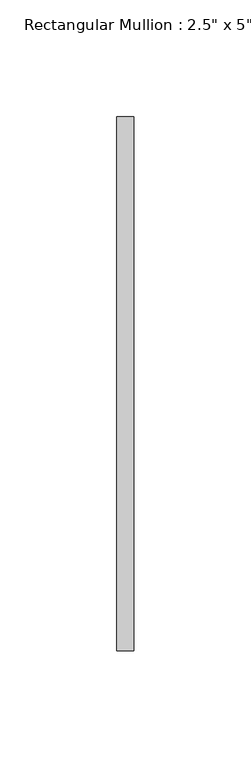
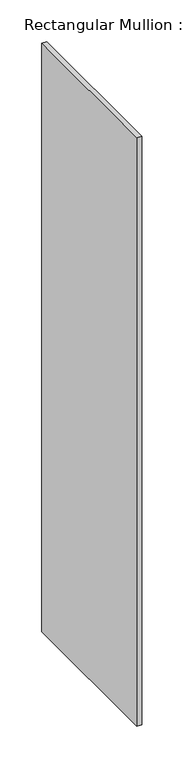
"""IFC4 building model written with IfcOpenShell, lengths in millimetres: member geometry."""

from ifc_helpers import new_model, si_unit, frame, origin, place, context, project, spatial, polyline, outline, extrude, source, transform, mapped, element, save


def member_049ff311(model_context):
    return source(origin(), model_context, "Body", "SweptSolid", [
        extrude(outline(polyline([(0.0, 114.3), (0.0, -114.3), (-7.239, -114.3), (-7.239, 114.3), (0.0, 114.3)])), frame((0.0, 0.0, -863.6), z_axis=(0.0, 0.0, 1.0), x_axis=(1.0, 0.0, 0.0)), (0.0, 0.0, 1.0), 863.6),
    ])


if __name__ == "__main__":
    model = new_model("IFC4")
    model_context = context("Model", 3, world=origin())
    ifc_project = project(units=[si_unit("LENGTHUNIT", "METRE", prefix="MILLI")], contexts=[model_context])
    site = spatial("IfcSite", under=ifc_project)
    building = spatial("IfcBuilding", under=site)
    placement = place(None, origin())
    member_shape = member_049ff311(model_context)
    element("IfcMember", 1, ObjectType="Rectangular Mullion : 2.5\" x 5\" rectangular", at=placement, inside=building, context=model_context, shape_type="MappedRepresentation", body=[
        mapped(member_shape, transform((0.0, 0.0, 0.0), x_axis=(1.0, 0.0, 0.0), y_axis=(0.0, 1.0, 0.0), z_axis=(0.0, 0.0, 1.0))),
    ])
    save(model, "model.ifc")

# Revit data of these elements
# Type "Rectangular Mullion : 2.5\" x 5\" rectangular"
#   built-in parameter 1007304 = 0.75 (stored number, unit not read)
#   built-in parameter 1007301 = 0.011875 (stored number, unit not read)
#   built-in parameter 1007300 = 0.011875 (stored number, unit not read)
# Element 1 (IfcMember, "Rectangular Mullion : 2.5\" x 5\" rectangular")
#   Materials on its faces: "WINDOW GLASS MATERIAL"
# Materials
#   "WINDOW GLASS MATERIAL": class "Generic", colour RGB 120 120 120, transparency 0, Cost = 0
